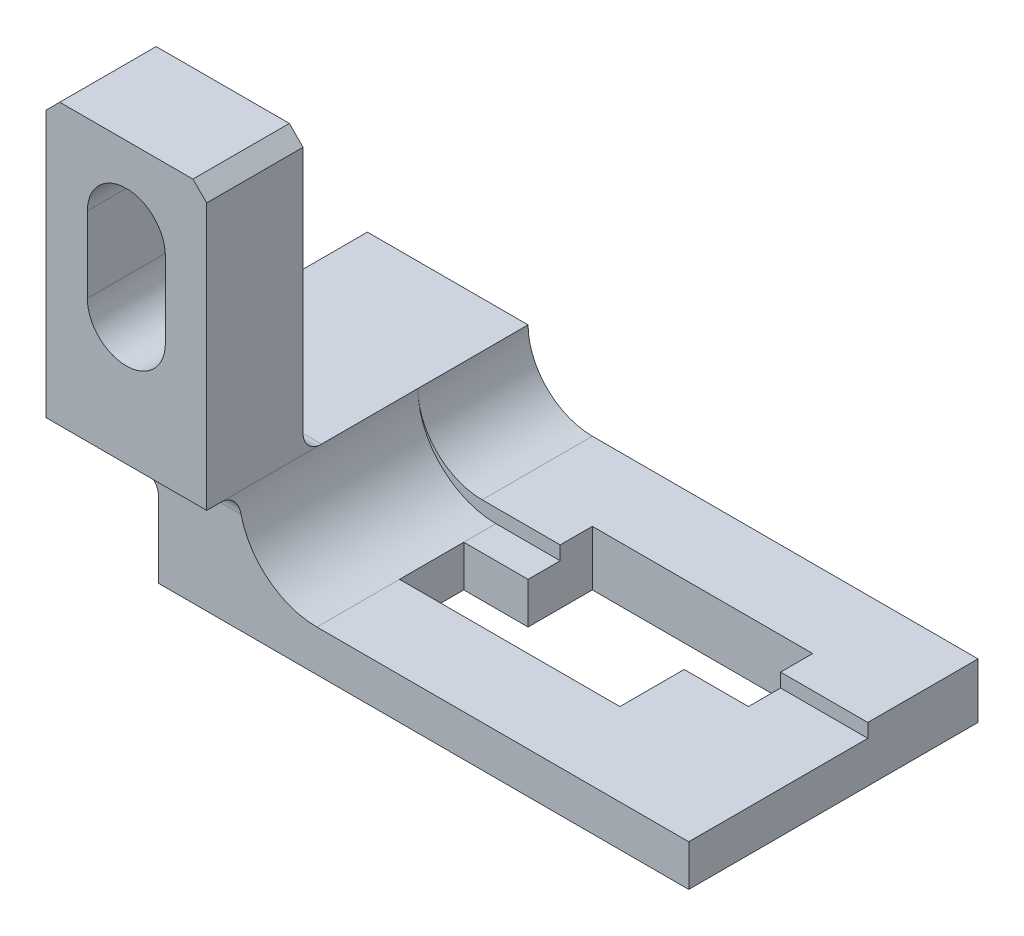
ISO-10303-21;
HEADER;
FILE_DESCRIPTION(('STEP AP214'),'2;1');
FILE_NAME('part.step','',(''),(''),'','','');
FILE_SCHEMA(('AUTOMOTIVE_DESIGN { 1 0 10303 214 1 1 1 1 }'));
ENDSEC;
DATA;
#1=APPLICATION_CONTEXT('core data for automotive mechanical design processes');
#2=APPLICATION_PROTOCOL_DEFINITION('international standard','automotive_design',2000,#1);
#3=PRODUCT_CONTEXT('',#1,'mechanical');
#4=PRODUCT('Part','Part','',(#3));
#5=PRODUCT_RELATED_PRODUCT_CATEGORY('part','',(#4));
#6=PRODUCT_DEFINITION_FORMATION('','',#4);
#7=PRODUCT_DEFINITION_CONTEXT('part definition',#1,'design');
#8=PRODUCT_DEFINITION('design','',#6,#7);
#9=PRODUCT_DEFINITION_SHAPE('','',#8);
#10=(LENGTH_UNIT() NAMED_UNIT(*) SI_UNIT(.MILLI.,.METRE.));
#11=(NAMED_UNIT(*) PLANE_ANGLE_UNIT() SI_UNIT($,.RADIAN.));
#12=(NAMED_UNIT(*) SI_UNIT($,.STERADIAN.) SOLID_ANGLE_UNIT());
#13=UNCERTAINTY_MEASURE_WITH_UNIT(LENGTH_MEASURE(1.E-05),#10,'distance_accuracy_value','');
#14=(GEOMETRIC_REPRESENTATION_CONTEXT(3) GLOBAL_UNCERTAINTY_ASSIGNED_CONTEXT((#13)) GLOBAL_UNIT_ASSIGNED_CONTEXT((#10,
#11,#12)) REPRESENTATION_CONTEXT('',''));
#15=CARTESIAN_POINT('',(0.,0.,0.));
#16=DIRECTION('',(0.,0.,1.));
#17=DIRECTION('',(1.,0.,0.));
#18=AXIS2_PLACEMENT_3D('',#15,#16,#17);
#19=CARTESIAN_POINT('',(0.,0.,31.5));
#20=DIRECTION('',(0.,-1.,0.));
#21=DIRECTION('',(0.,0.,-1.));
#22=AXIS2_PLACEMENT_3D('',#19,#20,#21);
#23=PLANE('',#22);
#24=DIRECTION('',(0.,0.,-1.));
#25=VECTOR('',#24,1.);
#26=CARTESIAN_POINT('',(0.,0.,31.5));
#27=LINE('',#26,#25);
#28=CARTESIAN_POINT('',(0.,0.,13.5));
#29=VERTEX_POINT('',#28);
#30=CARTESIAN_POINT('',(0.,0.,-31.5));
#31=VERTEX_POINT('',#30);
#32=EDGE_CURVE('E438',#29,#31,#27,.T.);
#33=ORIENTED_EDGE('',*,*,#32,.F.);
#34=DIRECTION('',(-1.,0.,0.));
#35=VECTOR('',#34,1.);
#36=CARTESIAN_POINT('',(0.,0.,13.5));
#37=LINE('',#36,#35);
#38=CARTESIAN_POINT('',(35.,0.,13.5));
#39=VERTEX_POINT('',#38);
#40=EDGE_CURVE('E507',#29,#39,#37,.F.);
#41=ORIENTED_EDGE('',*,*,#40,.T.);
#42=DIRECTION('',(0.,0.,-1.));
#43=VECTOR('',#42,1.);
#44=CARTESIAN_POINT('',(35.,0.,31.5));
#45=LINE('',#44,#43);
#46=CARTESIAN_POINT('',(35.,0.,-7.5));
#47=VERTEX_POINT('',#46);
#48=EDGE_CURVE('E467',#39,#47,#45,.T.);
#49=ORIENTED_EDGE('',*,*,#48,.T.);
#50=CARTESIAN_POINT('',(35.,0.,-31.5));
#51=VERTEX_POINT('',#50);
#52=EDGE_CURVE('E462',#47,#51,#45,.T.);
#53=ORIENTED_EDGE('',*,*,#52,.T.);
#54=DIRECTION('',(-1.,0.,0.));
#55=VECTOR('',#54,1.);
#56=CARTESIAN_POINT('',(0.,0.,-31.5));
#57=LINE('',#56,#55);
#58=EDGE_CURVE('E428',#51,#31,#57,.T.);
#59=ORIENTED_EDGE('',*,*,#58,.T.);
#60=EDGE_LOOP('',(#33,#41,#49,#53,#59));
#61=FACE_BOUND('',#60,.T.);
#62=ADVANCED_FACE('F41',(#61),#23,.F.);
#63=CARTESIAN_POINT('',(133.,-17.,-7.5));
#64=DIRECTION('',(0.,-1.,0.));
#65=DIRECTION('',(1.,0.,0.));
#66=AXIS2_PLACEMENT_3D('',#63,#64,#65);
#67=PLANE('',#66);
#68=DIRECTION('',(-1.,0.,0.));
#69=VECTOR('',#68,1.);
#70=CARTESIAN_POINT('',(52.,-17.,-0.49999999999999));
#71=LINE('',#70,#69);
#72=CARTESIAN_POINT('',(66.,-17.,-0.499999999999991));
#73=VERTEX_POINT('',#72);
#74=CARTESIAN_POINT('',(52.,-17.,-0.49999999999999));
#75=VERTEX_POINT('',#74);
#76=EDGE_CURVE('E340',#73,#75,#71,.T.);
#77=ORIENTED_EDGE('',*,*,#76,.F.);
#78=DIRECTION('',(0.,0.,1.));
#79=VECTOR('',#78,1.);
#80=CARTESIAN_POINT('',(66.,-17.,-0.499999999999991));
#81=LINE('',#80,#79);
#82=CARTESIAN_POINT('',(66.,-17.,-7.5));
#83=VERTEX_POINT('',#82);
#84=EDGE_CURVE('E339',#83,#73,#81,.T.);
#85=ORIENTED_EDGE('',*,*,#84,.F.);
#86=DIRECTION('',(1.,0.,0.));
#87=VECTOR('',#86,1.);
#88=CARTESIAN_POINT('',(133.,-17.,-7.5));
#89=LINE('',#88,#87);
#90=CARTESIAN_POINT('',(52.,-17.,-7.5));
#91=VERTEX_POINT('',#90);
#92=EDGE_CURVE('E414',#91,#83,#89,.T.);
#93=ORIENTED_EDGE('',*,*,#92,.F.);
#94=DIRECTION('',(0.,0.,1.));
#95=VECTOR('',#94,1.);
#96=CARTESIAN_POINT('',(52.,-17.,-7.5));
#97=LINE('',#96,#95);
#98=EDGE_CURVE('E425',#91,#75,#97,.T.);
#99=ORIENTED_EDGE('',*,*,#98,.T.);
#100=EDGE_LOOP('',(#77,#85,#93,#99));
#101=FACE_BOUND('',#100,.T.);
#102=ADVANCED_FACE('F586',(#101),#67,.F.);
#103=CARTESIAN_POINT('',(49.,0.,-7.5));
#104=DIRECTION('',(0.,0.,1.));
#105=DIRECTION('',(1.,0.,0.));
#106=AXIS2_PLACEMENT_3D('',#103,#104,#105);
#107=PLANE('',#106);
#108=DIRECTION('',(0.,1.,0.));
#109=VECTOR('',#108,1.);
#110=CARTESIAN_POINT('',(66.,-26.001,-7.5));
#111=LINE('',#110,#109);
#112=CARTESIAN_POINT('',(66.,-14.,-7.5));
#113=VERTEX_POINT('',#112);
#114=EDGE_CURVE('E330',#83,#113,#111,.T.);
#115=ORIENTED_EDGE('',*,*,#114,.T.);
#116=DIRECTION('',(-1.,0.,0.));
#117=VECTOR('',#116,1.);
#118=CARTESIAN_POINT('',(133.,-14.,-7.5));
#119=LINE('',#118,#117);
#120=CARTESIAN_POINT('',(49.,-14.,-7.5));
#121=VERTEX_POINT('',#120);
#122=EDGE_CURVE('E398',#113,#121,#119,.T.);
#123=ORIENTED_EDGE('',*,*,#122,.T.);
#124=CARTESIAN_POINT('',(49.,0.,-7.5));
#125=DIRECTION('',(0.,0.,-1.));
#126=DIRECTION('',(1.,0.,0.));
#127=AXIS2_PLACEMENT_3D('',#124,#125,#126);
#128=CIRCLE('',#127,14.);
#129=EDGE_CURVE('E403',#121,#47,#128,.T.);
#130=ORIENTED_EDGE('',*,*,#129,.T.);
#131=CARTESIAN_POINT('',(52.,0.,-7.5));
#132=DIRECTION('',(0.,0.,1.));
#133=DIRECTION('',(-1.,0.,0.));
#134=AXIS2_PLACEMENT_3D('',#131,#132,#133);
#135=CIRCLE('',#134,17.);
#136=EDGE_CURVE('E409',#47,#91,#135,.T.);
#137=ORIENTED_EDGE('',*,*,#136,.T.);
#138=ORIENTED_EDGE('',*,*,#92,.T.);
#139=EDGE_LOOP('',(#115,#123,#130,#137,#138));
#140=FACE_BOUND('',#139,.T.);
#141=ADVANCED_FACE('F591',(#140),#107,.T.);
#142=CARTESIAN_POINT('',(49.,-14.,31.5));
#143=DIRECTION('',(0.,-1.,0.));
#144=DIRECTION('',(1.,0.,0.));
#145=AXIS2_PLACEMENT_3D('',#142,#143,#144);
#146=PLANE('',#145);
#147=ORIENTED_EDGE('',*,*,#122,.F.);
#148=DIRECTION('',(0.,0.,1.));
#149=VECTOR('',#148,1.);
#150=CARTESIAN_POINT('',(66.,-14.,-0.499999999999991));
#151=LINE('',#150,#149);
#152=CARTESIAN_POINT('',(66.,-14.,-14.5));
#153=VERTEX_POINT('',#152);
#154=EDGE_CURVE('E366',#153,#113,#151,.T.);
#155=ORIENTED_EDGE('',*,*,#154,.F.);
#156=DIRECTION('',(-1.,0.,0.));
#157=VECTOR('',#156,1.);
#158=CARTESIAN_POINT('',(66.,-14.,-14.5));
#159=LINE('',#158,#157);
#160=CARTESIAN_POINT('',(114.,-14.,-14.5));
#161=VERTEX_POINT('',#160);
#162=EDGE_CURVE('E364',#161,#153,#159,.T.);
#163=ORIENTED_EDGE('',*,*,#162,.F.);
#164=DIRECTION('',(0.,0.,-1.));
#165=VECTOR('',#164,1.);
#166=CARTESIAN_POINT('',(114.,-14.,-14.5));
#167=LINE('',#166,#165);
#168=CARTESIAN_POINT('',(114.,-14.,-7.5));
#169=VERTEX_POINT('',#168);
#170=EDGE_CURVE('E362',#169,#161,#167,.T.);
#171=ORIENTED_EDGE('',*,*,#170,.F.);
#172=CARTESIAN_POINT('',(133.,-14.,-7.5));
#173=VERTEX_POINT('',#172);
#174=EDGE_CURVE('E405',#173,#169,#119,.T.);
#175=ORIENTED_EDGE('',*,*,#174,.F.);
#176=DIRECTION('',(0.,0.,-1.));
#177=VECTOR('',#176,1.);
#178=CARTESIAN_POINT('',(133.,-14.,31.5));
#179=LINE('',#178,#177);
#180=CARTESIAN_POINT('',(133.,-14.,-31.5));
#181=VERTEX_POINT('',#180);
#182=EDGE_CURVE('E470',#173,#181,#179,.T.);
#183=ORIENTED_EDGE('',*,*,#182,.T.);
#184=DIRECTION('',(-1.,0.,0.));
#185=VECTOR('',#184,1.);
#186=CARTESIAN_POINT('',(49.,-14.,-31.5));
#187=LINE('',#186,#185);
#188=CARTESIAN_POINT('',(49.,-14.,-31.5));
#189=VERTEX_POINT('',#188);
#190=EDGE_CURVE('E455',#181,#189,#187,.T.);
#191=ORIENTED_EDGE('',*,*,#190,.T.);
#192=DIRECTION('',(0.,0.,-1.));
#193=VECTOR('',#192,1.);
#194=CARTESIAN_POINT('',(49.,-14.,31.5));
#195=LINE('',#194,#193);
#196=EDGE_CURVE('E465',#121,#189,#195,.T.);
#197=ORIENTED_EDGE('',*,*,#196,.F.);
#198=EDGE_LOOP('',(#147,#155,#163,#171,#175,#183,#191,#197));
#199=FACE_BOUND('',#198,.T.);
#200=ADVANCED_FACE('F557',(#199),#146,.F.);
#201=CARTESIAN_POINT('',(49.,0.,31.5));
#202=DIRECTION('',(0.,0.,-1.));
#203=DIRECTION('',(-1.,0.,0.));
#204=AXIS2_PLACEMENT_3D('',#201,#202,#203);
#205=CYLINDRICAL_SURFACE('',#204,14.);
#206=ORIENTED_EDGE('',*,*,#129,.F.);
#207=ORIENTED_EDGE('',*,*,#196,.T.);
#208=CARTESIAN_POINT('',(49.,0.,-31.5));
#209=DIRECTION('',(0.,0.,-1.));
#210=DIRECTION('',(1.,0.,0.));
#211=AXIS2_PLACEMENT_3D('',#208,#209,#210);
#212=CIRCLE('',#211,14.);
#213=EDGE_CURVE('E457',#189,#51,#212,.T.);
#214=ORIENTED_EDGE('',*,*,#213,.T.);
#215=ORIENTED_EDGE('',*,*,#52,.F.);
#216=EDGE_LOOP('',(#206,#207,#214,#215));
#217=FACE_BOUND('',#216,.T.);
#218=ADVANCED_FACE('F648',(#217),#205,.F.);
#219=CARTESIAN_POINT('',(0.,0.,31.5));
#220=DIRECTION('',(1.,0.,0.));
#221=DIRECTION('',(0.,1.,0.));
#222=AXIS2_PLACEMENT_3D('',#219,#220,#221);
#223=PLANE('',#222);
#224=DIRECTION('',(0.,1.,0.));
#225=VECTOR('',#224,1.);
#226=CARTESIAN_POINT('',(0.,0.,38.5));
#227=LINE('',#226,#225);
#228=CARTESIAN_POINT('',(0.,0.,38.5));
#229=VERTEX_POINT('',#228);
#230=CARTESIAN_POINT('',(0.,58.,38.5));
#231=VERTEX_POINT('',#230);
#232=EDGE_CURVE('E301',#229,#231,#227,.T.);
#233=ORIENTED_EDGE('',*,*,#232,.T.);
#234=DIRECTION('',(0.,0.,-1.));
#235=VECTOR('',#234,1.);
#236=CARTESIAN_POINT('',(0.,58.,17.5));
#237=LINE('',#236,#235);
#238=CARTESIAN_POINT('',(0.,58.,17.5));
#239=VERTEX_POINT('',#238);
#240=EDGE_CURVE('E484',#231,#239,#237,.T.);
#241=ORIENTED_EDGE('',*,*,#240,.T.);
#242=DIRECTION('',(0.,-1.,0.));
#243=VECTOR('',#242,1.);
#244=CARTESIAN_POINT('',(0.,61.,17.5));
#245=LINE('',#244,#243);
#246=CARTESIAN_POINT('',(0.,4.,17.5));
#247=VERTEX_POINT('',#246);
#248=EDGE_CURVE('E298',#239,#247,#245,.T.);
#249=ORIENTED_EDGE('',*,*,#248,.T.);
#250=CARTESIAN_POINT('',(0.,4.,13.5));
#251=DIRECTION('',(1.,0.,0.));
#252=DIRECTION('',(0.,1.,0.));
#253=AXIS2_PLACEMENT_3D('',#250,#251,#252);
#254=CIRCLE('',#253,4.);
#255=EDGE_CURVE('E513',#247,#29,#254,.T.);
#256=ORIENTED_EDGE('',*,*,#255,.T.);
#257=ORIENTED_EDGE('',*,*,#32,.T.);
#258=DIRECTION('',(0.,-1.,0.));
#259=VECTOR('',#258,1.);
#260=CARTESIAN_POINT('',(0.,0.,-31.5));
#261=LINE('',#260,#259);
#262=CARTESIAN_POINT('',(0.,-6.,-31.5));
#263=VERTEX_POINT('',#262);
#264=EDGE_CURVE('E423',#31,#263,#261,.T.);
#265=ORIENTED_EDGE('',*,*,#264,.T.);
#266=DIRECTION('',(0.,0.,-1.));
#267=VECTOR('',#266,1.);
#268=CARTESIAN_POINT('',(0.,-6.,31.5));
#269=LINE('',#268,#267);
#270=CARTESIAN_POINT('',(0.,-6.,31.5));
#271=VERTEX_POINT('',#270);
#272=EDGE_CURVE('E485',#271,#263,#269,.T.);
#273=ORIENTED_EDGE('',*,*,#272,.F.);
#274=DIRECTION('',(0.,-1.,0.));
#275=VECTOR('',#274,1.);
#276=CARTESIAN_POINT('',(0.,0.,31.5));
#277=LINE('',#276,#275);
#278=CARTESIAN_POINT('',(0.,-4.,31.5));
#279=VERTEX_POINT('',#278);
#280=EDGE_CURVE('E422',#279,#271,#277,.T.);
#281=ORIENTED_EDGE('',*,*,#280,.F.);
#282=CARTESIAN_POINT('',(0.,-4.,35.5));
#283=DIRECTION('',(1.,0.,0.));
#284=DIRECTION('',(0.,1.,0.));
#285=AXIS2_PLACEMENT_3D('',#282,#283,#284);
#286=CIRCLE('',#285,4.);
#287=CARTESIAN_POINT('',(0.,0.,35.5));
#288=VERTEX_POINT('',#287);
#289=EDGE_CURVE('E54',#279,#288,#286,.T.);
#290=ORIENTED_EDGE('',*,*,#289,.T.);
#291=DIRECTION('',(0.,0.,1.));
#292=VECTOR('',#291,1.);
#293=CARTESIAN_POINT('',(0.,0.,17.5));
#294=LINE('',#293,#292);
#295=EDGE_CURVE('E315',#288,#229,#294,.T.);
#296=ORIENTED_EDGE('',*,*,#295,.T.);
#297=EDGE_LOOP('',(#233,#241,#249,#256,#257,#265,#273,#281,#290,#296));
#298=FACE_BOUND('',#297,.T.);
#299=ADVANCED_FACE('F522',(#298),#223,.F.);
#300=CARTESIAN_POINT('',(0.,-6.,31.5));
#301=DIRECTION('',(0.,1.,0.));
#302=DIRECTION('',(0.,0.,1.));
#303=AXIS2_PLACEMENT_3D('',#300,#301,#302);
#304=PLANE('',#303);
#305=DIRECTION('',(1.,0.,0.));
#306=VECTOR('',#305,1.);
#307=CARTESIAN_POINT('',(0.,-6.,-31.5));
#308=LINE('',#307,#306);
#309=CARTESIAN_POINT('',(14.,-6.,-31.5));
#310=VERTEX_POINT('',#309);
#311=EDGE_CURVE('E445',#263,#310,#308,.T.);
#312=ORIENTED_EDGE('',*,*,#311,.T.);
#313=DIRECTION('',(0.,0.,-1.));
#314=VECTOR('',#313,1.);
#315=CARTESIAN_POINT('',(14.,-6.,31.5));
#316=LINE('',#315,#314);
#317=CARTESIAN_POINT('',(14.,-6.,31.5));
#318=VERTEX_POINT('',#317);
#319=EDGE_CURVE('E479',#318,#310,#316,.T.);
#320=ORIENTED_EDGE('',*,*,#319,.F.);
#321=DIRECTION('',(1.,0.,0.));
#322=VECTOR('',#321,1.);
#323=CARTESIAN_POINT('',(0.,-6.,31.5));
#324=LINE('',#323,#322);
#325=EDGE_CURVE('E430',#271,#318,#324,.T.);
#326=ORIENTED_EDGE('',*,*,#325,.F.);
#327=ORIENTED_EDGE('',*,*,#272,.T.);
#328=EDGE_LOOP('',(#312,#320,#326,#327));
#329=FACE_BOUND('',#328,.T.);
#330=ADVANCED_FACE('F630',(#329),#304,.F.);
#331=CARTESIAN_POINT('',(14.,-9.5,31.5));
#332=DIRECTION('',(0.,0.,-1.));
#333=DIRECTION('',(-1.,0.,0.));
#334=AXIS2_PLACEMENT_3D('',#331,#332,#333);
#335=CYLINDRICAL_SURFACE('',#334,3.5);
#336=CARTESIAN_POINT('',(14.,-9.5,-31.5));
#337=DIRECTION('',(0.,0.,-1.));
#338=DIRECTION('',(-1.,0.,0.));
#339=AXIS2_PLACEMENT_3D('',#336,#337,#338);
#340=CIRCLE('',#339,3.5);
#341=CARTESIAN_POINT('',(17.5,-9.50000000000002,-31.5));
#342=VERTEX_POINT('',#341);
#343=EDGE_CURVE('E441',#310,#342,#340,.T.);
#344=ORIENTED_EDGE('',*,*,#343,.T.);
#345=DIRECTION('',(0.,0.,-1.));
#346=VECTOR('',#345,1.);
#347=CARTESIAN_POINT('',(17.5,-9.50000000000002,31.5));
#348=LINE('',#347,#346);
#349=CARTESIAN_POINT('',(17.5,-9.50000000000002,31.5));
#350=VERTEX_POINT('',#349);
#351=EDGE_CURVE('E478',#350,#342,#348,.T.);
#352=ORIENTED_EDGE('',*,*,#351,.F.);
#353=CARTESIAN_POINT('',(14.,-9.5,31.5));
#354=DIRECTION('',(0.,0.,-1.));
#355=DIRECTION('',(-1.,0.,0.));
#356=AXIS2_PLACEMENT_3D('',#353,#354,#355);
#357=CIRCLE('',#356,3.5);
#358=EDGE_CURVE('E429',#318,#350,#357,.T.);
#359=ORIENTED_EDGE('',*,*,#358,.F.);
#360=ORIENTED_EDGE('',*,*,#319,.T.);
#361=EDGE_LOOP('',(#344,#352,#359,#360));
#362=FACE_BOUND('',#361,.T.);
#363=ADVANCED_FACE('F637',(#362),#335,.F.);
#364=CARTESIAN_POINT('',(17.5,-9.50000000000002,31.5));
#365=DIRECTION('',(1.,0.,0.));
#366=DIRECTION('',(0.,1.,0.));
#367=AXIS2_PLACEMENT_3D('',#364,#365,#366);
#368=PLANE('',#367);
#369=DIRECTION('',(0.,-1.,0.));
#370=VECTOR('',#369,1.);
#371=CARTESIAN_POINT('',(17.5,-9.50000000000002,-31.5));
#372=LINE('',#371,#370);
#373=CARTESIAN_POINT('',(17.5,-26.,-31.5));
#374=VERTEX_POINT('',#373);
#375=EDGE_CURVE('E446',#342,#374,#372,.T.);
#376=ORIENTED_EDGE('',*,*,#375,.T.);
#377=DIRECTION('',(0.,0.,-1.));
#378=VECTOR('',#377,1.);
#379=CARTESIAN_POINT('',(17.5,-26.,31.5));
#380=LINE('',#379,#378);
#381=CARTESIAN_POINT('',(17.5,-26.,31.5));
#382=VERTEX_POINT('',#381);
#383=EDGE_CURVE('E471',#382,#374,#380,.T.);
#384=ORIENTED_EDGE('',*,*,#383,.F.);
#385=DIRECTION('',(0.,-1.,0.));
#386=VECTOR('',#385,1.);
#387=CARTESIAN_POINT('',(17.5,-9.50000000000002,31.5));
#388=LINE('',#387,#386);
#389=EDGE_CURVE('E435',#350,#382,#388,.T.);
#390=ORIENTED_EDGE('',*,*,#389,.F.);
#391=ORIENTED_EDGE('',*,*,#351,.T.);
#392=EDGE_LOOP('',(#376,#384,#390,#391));
#393=FACE_BOUND('',#392,.T.);
#394=ADVANCED_FACE('F639',(#393),#368,.F.);
#395=CARTESIAN_POINT('',(133.,-26.,31.5));
#396=DIRECTION('',(0.,1.,0.));
#397=DIRECTION('',(0.,0.,1.));
#398=AXIS2_PLACEMENT_3D('',#395,#396,#397);
#399=PLANE('',#398);
#400=DIRECTION('',(0.,0.,-1.));
#401=VECTOR('',#400,1.);
#402=CARTESIAN_POINT('',(66.,-26.,-0.499999999999991));
#403=LINE('',#402,#401);
#404=CARTESIAN_POINT('',(66.,-26.,-0.499999999999991));
#405=VERTEX_POINT('',#404);
#406=CARTESIAN_POINT('',(66.,-26.,-14.5));
#407=VERTEX_POINT('',#406);
#408=EDGE_CURVE('E357',#405,#407,#403,.T.);
#409=ORIENTED_EDGE('',*,*,#408,.F.);
#410=DIRECTION('',(1.,0.,0.));
#411=VECTOR('',#410,1.);
#412=CARTESIAN_POINT('',(52.,-26.,-0.49999999999999));
#413=LINE('',#412,#411);
#414=CARTESIAN_POINT('',(52.,-26.,-0.49999999999999));
#415=VERTEX_POINT('',#414);
#416=EDGE_CURVE('E356',#415,#405,#413,.T.);
#417=ORIENTED_EDGE('',*,*,#416,.F.);
#418=DIRECTION('',(0.,0.,-1.));
#419=VECTOR('',#418,1.);
#420=CARTESIAN_POINT('',(52.,-26.,13.5));
#421=LINE('',#420,#419);
#422=CARTESIAN_POINT('',(52.,-26.,13.5));
#423=VERTEX_POINT('',#422);
#424=EDGE_CURVE('E393',#423,#415,#421,.T.);
#425=ORIENTED_EDGE('',*,*,#424,.F.);
#426=DIRECTION('',(-1.,0.,0.));
#427=VECTOR('',#426,1.);
#428=CARTESIAN_POINT('',(100.,-26.,13.5));
#429=LINE('',#428,#427);
#430=CARTESIAN_POINT('',(100.,-26.,13.5));
#431=VERTEX_POINT('',#430);
#432=EDGE_CURVE('E344',#431,#423,#429,.T.);
#433=ORIENTED_EDGE('',*,*,#432,.F.);
#434=DIRECTION('',(0.,0.,1.));
#435=VECTOR('',#434,1.);
#436=CARTESIAN_POINT('',(100.,-26.,-0.499999999999997));
#437=LINE('',#436,#435);
#438=CARTESIAN_POINT('',(100.,-26.,-0.499999999999997));
#439=VERTEX_POINT('',#438);
#440=EDGE_CURVE('E343',#439,#431,#437,.T.);
#441=ORIENTED_EDGE('',*,*,#440,.F.);
#442=DIRECTION('',(-1.,0.,0.));
#443=VECTOR('',#442,1.);
#444=CARTESIAN_POINT('',(114.,-26.,-0.499999999999999));
#445=LINE('',#444,#443);
#446=CARTESIAN_POINT('',(114.,-26.,-0.499999999999999));
#447=VERTEX_POINT('',#446);
#448=EDGE_CURVE('E350',#447,#439,#445,.T.);
#449=ORIENTED_EDGE('',*,*,#448,.F.);
#450=DIRECTION('',(0.,0.,1.));
#451=VECTOR('',#450,1.);
#452=CARTESIAN_POINT('',(114.,-26.,-14.5));
#453=LINE('',#452,#451);
#454=CARTESIAN_POINT('',(114.,-26.,-14.5));
#455=VERTEX_POINT('',#454);
#456=EDGE_CURVE('E348',#455,#447,#453,.T.);
#457=ORIENTED_EDGE('',*,*,#456,.F.);
#458=DIRECTION('',(1.,0.,0.));
#459=VECTOR('',#458,1.);
#460=CARTESIAN_POINT('',(66.,-26.,-14.5));
#461=LINE('',#460,#459);
#462=EDGE_CURVE('E354',#407,#455,#461,.T.);
#463=ORIENTED_EDGE('',*,*,#462,.F.);
#464=EDGE_LOOP('',(#409,#417,#425,#433,#441,#449,#457,#463));
#465=FACE_BOUND('',#464,.T.);
#466=DIRECTION('',(1.,0.,0.));
#467=VECTOR('',#466,1.);
#468=CARTESIAN_POINT('',(133.,-26.,-31.5));
#469=LINE('',#468,#467);
#470=CARTESIAN_POINT('',(133.,-26.,-31.5));
#471=VERTEX_POINT('',#470);
#472=EDGE_CURVE('E449',#374,#471,#469,.T.);
#473=ORIENTED_EDGE('',*,*,#472,.T.);
#474=DIRECTION('',(0.,0.,-1.));
#475=VECTOR('',#474,1.);
#476=CARTESIAN_POINT('',(133.,-26.,31.5));
#477=LINE('',#476,#475);
#478=CARTESIAN_POINT('',(133.,-26.,31.5));
#479=VERTEX_POINT('',#478);
#480=EDGE_CURVE('E468',#479,#471,#477,.T.);
#481=ORIENTED_EDGE('',*,*,#480,.F.);
#482=DIRECTION('',(1.,0.,0.));
#483=VECTOR('',#482,1.);
#484=CARTESIAN_POINT('',(133.,-26.,31.5));
#485=LINE('',#484,#483);
#486=EDGE_CURVE('E432',#382,#479,#485,.T.);
#487=ORIENTED_EDGE('',*,*,#486,.F.);
#488=ORIENTED_EDGE('',*,*,#383,.T.);
#489=EDGE_LOOP('',(#473,#481,#487,#488));
#490=FACE_BOUND('',#489,.T.);
#491=ADVANCED_FACE('F574',(#465,#490),#399,.F.);
#492=CARTESIAN_POINT('',(133.,-14.,31.5));
#493=DIRECTION('',(-1.,0.,0.));
#494=DIRECTION('',(0.,0.,1.));
#495=AXIS2_PLACEMENT_3D('',#492,#493,#494);
#496=PLANE('',#495);
#497=DIRECTION('',(0.,1.,0.));
#498=VECTOR('',#497,1.);
#499=CARTESIAN_POINT('',(133.,-17.,-7.5));
#500=LINE('',#499,#498);
#501=CARTESIAN_POINT('',(133.,-17.,-7.5));
#502=VERTEX_POINT('',#501);
#503=EDGE_CURVE('E400',#502,#173,#500,.T.);
#504=ORIENTED_EDGE('',*,*,#503,.F.);
#505=DIRECTION('',(0.,0.,1.));
#506=VECTOR('',#505,1.);
#507=CARTESIAN_POINT('',(133.,-17.,-7.5));
#508=LINE('',#507,#506);
#509=CARTESIAN_POINT('',(133.,-17.,31.5));
#510=VERTEX_POINT('',#509);
#511=EDGE_CURVE('E416',#502,#510,#508,.T.);
#512=ORIENTED_EDGE('',*,*,#511,.T.);
#513=DIRECTION('',(0.,1.,0.));
#514=VECTOR('',#513,1.);
#515=CARTESIAN_POINT('',(133.,-14.,31.5));
#516=LINE('',#515,#514);
#517=EDGE_CURVE('E436',#479,#510,#516,.T.);
#518=ORIENTED_EDGE('',*,*,#517,.F.);
#519=ORIENTED_EDGE('',*,*,#480,.T.);
#520=DIRECTION('',(0.,1.,0.));
#521=VECTOR('',#520,1.);
#522=CARTESIAN_POINT('',(133.,-14.,-31.5));
#523=LINE('',#522,#521);
#524=EDGE_CURVE('E450',#471,#181,#523,.T.);
#525=ORIENTED_EDGE('',*,*,#524,.T.);
#526=ORIENTED_EDGE('',*,*,#182,.F.);
#527=EDGE_LOOP('',(#504,#512,#518,#519,#525,#526));
#528=FACE_BOUND('',#527,.T.);
#529=ADVANCED_FACE('F548',(#528),#496,.F.);
#530=CARTESIAN_POINT('',(14.,-9.5,31.5));
#531=DIRECTION('',(0.,0.,-1.));
#532=DIRECTION('',(-1.,0.,0.));
#533=AXIS2_PLACEMENT_3D('',#530,#531,#532);
#534=PLANE('',#533);
#535=CARTESIAN_POINT('',(52.,0.,31.5));
#536=DIRECTION('',(0.,0.,1.));
#537=DIRECTION('',(-1.,0.,0.));
#538=AXIS2_PLACEMENT_3D('',#535,#536,#537);
#539=CIRCLE('',#538,17.);
#540=CARTESIAN_POINT('',(35.4772883581417,-4.,31.5));
#541=VERTEX_POINT('',#540);
#542=CARTESIAN_POINT('',(52.,-17.,31.5));
#543=VERTEX_POINT('',#542);
#544=EDGE_CURVE('E399',#541,#543,#539,.T.);
#545=ORIENTED_EDGE('',*,*,#544,.F.);
#546=DIRECTION('',(-1.,0.,0.));
#547=VECTOR('',#546,1.);
#548=CARTESIAN_POINT('',(14.,-4.,31.5));
#549=LINE('',#548,#547);
#550=EDGE_CURVE('E506',#541,#279,#549,.T.);
#551=ORIENTED_EDGE('',*,*,#550,.T.);
#552=ORIENTED_EDGE('',*,*,#280,.T.);
#553=ORIENTED_EDGE('',*,*,#325,.T.);
#554=ORIENTED_EDGE('',*,*,#358,.T.);
#555=ORIENTED_EDGE('',*,*,#389,.T.);
#556=ORIENTED_EDGE('',*,*,#486,.T.);
#557=ORIENTED_EDGE('',*,*,#517,.T.);
#558=DIRECTION('',(1.,0.,0.));
#559=VECTOR('',#558,1.);
#560=CARTESIAN_POINT('',(133.,-17.,31.5));
#561=LINE('',#560,#559);
#562=EDGE_CURVE('E402',#543,#510,#561,.T.);
#563=ORIENTED_EDGE('',*,*,#562,.F.);
#564=EDGE_LOOP('',(#545,#551,#552,#553,#554,#555,#556,#557,#563));
#565=FACE_BOUND('',#564,.T.);
#566=ADVANCED_FACE('F539',(#565),#534,.F.);
#567=CARTESIAN_POINT('',(14.,-9.5,-31.5));
#568=DIRECTION('',(0.,0.,-1.));
#569=DIRECTION('',(-1.,0.,0.));
#570=AXIS2_PLACEMENT_3D('',#567,#568,#569);
#571=PLANE('',#570);
#572=ORIENTED_EDGE('',*,*,#264,.F.);
#573=ORIENTED_EDGE('',*,*,#58,.F.);
#574=ORIENTED_EDGE('',*,*,#213,.F.);
#575=ORIENTED_EDGE('',*,*,#190,.F.);
#576=ORIENTED_EDGE('',*,*,#524,.F.);
#577=ORIENTED_EDGE('',*,*,#472,.F.);
#578=ORIENTED_EDGE('',*,*,#375,.F.);
#579=ORIENTED_EDGE('',*,*,#343,.F.);
#580=ORIENTED_EDGE('',*,*,#311,.F.);
#581=EDGE_LOOP('',(#572,#573,#574,#575,#576,#577,#578,#579,#580));
#582=FACE_BOUND('',#581,.T.);
#583=ADVANCED_FACE('F626',(#582),#571,.T.);
#584=CARTESIAN_POINT('',(114.,-17.,-7.5));
#585=VERTEX_POINT('',#584);
#586=EDGE_CURVE('E412',#585,#502,#89,.T.);
#587=ORIENTED_EDGE('',*,*,#586,.F.);
#588=DIRECTION('',(0.,0.,-1.));
#589=VECTOR('',#588,1.);
#590=CARTESIAN_POINT('',(114.,-17.,-14.5));
#591=LINE('',#590,#589);
#592=CARTESIAN_POINT('',(114.,-17.,-0.499999999999999));
#593=VERTEX_POINT('',#592);
#594=EDGE_CURVE('E336',#593,#585,#591,.T.);
#595=ORIENTED_EDGE('',*,*,#594,.F.);
#596=DIRECTION('',(1.,0.,0.));
#597=VECTOR('',#596,1.);
#598=CARTESIAN_POINT('',(114.,-17.,-0.499999999999999));
#599=LINE('',#598,#597);
#600=CARTESIAN_POINT('',(100.,-17.,-0.499999999999997));
#601=VERTEX_POINT('',#600);
#602=EDGE_CURVE('E331',#601,#593,#599,.T.);
#603=ORIENTED_EDGE('',*,*,#602,.F.);
#604=DIRECTION('',(0.,0.,-1.));
#605=VECTOR('',#604,1.);
#606=CARTESIAN_POINT('',(100.,-17.,-0.499999999999997));
#607=LINE('',#606,#605);
#608=CARTESIAN_POINT('',(100.,-17.,13.5));
#609=VERTEX_POINT('',#608);
#610=EDGE_CURVE('E335',#609,#601,#607,.T.);
#611=ORIENTED_EDGE('',*,*,#610,.F.);
#612=DIRECTION('',(1.,0.,0.));
#613=VECTOR('',#612,1.);
#614=CARTESIAN_POINT('',(100.,-17.,13.5));
#615=LINE('',#614,#613);
#616=CARTESIAN_POINT('',(52.,-17.,13.5));
#617=VERTEX_POINT('',#616);
#618=EDGE_CURVE('E329',#617,#609,#615,.T.);
#619=ORIENTED_EDGE('',*,*,#618,.F.);
#620=EDGE_CURVE('E413',#617,#543,#97,.T.);
#621=ORIENTED_EDGE('',*,*,#620,.T.);
#622=ORIENTED_EDGE('',*,*,#562,.T.);
#623=ORIENTED_EDGE('',*,*,#511,.F.);
#624=EDGE_LOOP('',(#587,#595,#603,#611,#619,#621,#622,#623));
#625=FACE_BOUND('',#624,.T.);
#626=ADVANCED_FACE('F544',(#625),#67,.F.);
#627=CARTESIAN_POINT('',(52.,0.,-7.5));
#628=DIRECTION('',(0.,0.,1.));
#629=DIRECTION('',(1.,0.,0.));
#630=AXIS2_PLACEMENT_3D('',#627,#628,#629);
#631=CYLINDRICAL_SURFACE('',#630,17.);
#632=CARTESIAN_POINT('',(35.,0.,35.5));
#633=VERTEX_POINT('',#632);
#634=EDGE_CURVE('E464',#633,#39,#45,.T.);
#635=ORIENTED_EDGE('',*,*,#634,.F.);
#636=CARTESIAN_POINT('',(35.,0.,35.5));
#637=CARTESIAN_POINT('',(35.0000083013039,1.07492089478438E-05,35.3875551600864));
#638=CARTESIAN_POINT('',(35.0000002164993,-0.00474140518274543,35.2751154336279));
#639=CARTESIAN_POINT('',(35.0000116692192,-0.0236883223681302,35.0510393368197));
#640=CARTESIAN_POINT('',(35.0000312054831,-0.0378826542354126,34.9394029300426));
#641=CARTESIAN_POINT('',(35.0001582427405,-0.0756183018738792,34.717789251689));
#642=CARTESIAN_POINT('',(35.0002656857482,-0.0991534509001617,34.6078109350756));
#643=CARTESIAN_POINT('',(35.0006870800331,-0.155379787783206,34.3902538389751));
#644=CARTESIAN_POINT('',(35.0010010287807,-0.188070863480572,34.2826750301115));
#645=CARTESIAN_POINT('',(35.002475089407,-0.299616249295769,33.9645689947982));
#646=CARTESIAN_POINT('',(35.0041672532816,-0.391956983501848,33.7585888256198));
#647=CARTESIAN_POINT('',(35.0105940252902,-0.609815982718297,33.3652251157232));
#648=CARTESIAN_POINT('',(35.0153281210827,-0.73532865860424,33.1778384495034));
#649=CARTESIAN_POINT('',(35.0297860201258,-1.01559300260569,32.8272621179482));
#650=CARTESIAN_POINT('',(35.039498240105,-1.17027626977358,32.6640174094866));
#651=CARTESIAN_POINT('',(35.0658728098731,-1.50444396712971,32.3659410961021));
#652=CARTESIAN_POINT('',(35.0825349222226,-1.68392754988818,32.2311085207306));
#653=CARTESIAN_POINT('',(35.1242644518129,-2.06034746483842,31.9947635630701));
#654=CARTESIAN_POINT('',(35.1492509862175,-2.25710292450681,31.8929484702819));
#655=CARTESIAN_POINT('',(35.2086941877631,-2.66348109747532,31.7234753466681));
#656=CARTESIAN_POINT('',(35.2431488829303,-2.87310112436463,31.6558102116013));
#657=CARTESIAN_POINT('',(35.310239320715,-3.23657295611819,31.5704717798367));
#658=CARTESIAN_POINT('',(35.3404773885729,-3.38886856149081,31.5439754018867));
#659=CARTESIAN_POINT('',(35.405514535937,-3.69427664557593,31.5087371885203));
#660=CARTESIAN_POINT('',(35.4403060702223,-3.84738737956684,31.4999663682107));
#661=CARTESIAN_POINT('',(35.4772883581417,-4.,31.5));
#662=B_SPLINE_CURVE_WITH_KNOTS('',3,(#636,#637,#638,#639,#640,#641,#642,#643,#644,#645,#646,
#647,#648,#649,#650,#651,#652,#653,#654,#655,#656,#657,#658,#659,#660,#661),.UNSPECIFIED.,.F.,
.F.,(4,2,2,2,2,2,2,2,2,2,2,2,4),(0.,0.337224909482972,0.674434429597278,1.01142169557896,
1.34840483367311,2.02212066534948,2.69572305525769,3.36776515140771,4.0397842894742,
4.70545556424118,5.37098830177873,5.8425107249983,6.31326148722317),.UNSPECIFIED.);
#663=EDGE_CURVE('E11',#633,#541,#662,.T.);
#664=ORIENTED_EDGE('',*,*,#663,.T.);
#665=ORIENTED_EDGE('',*,*,#544,.T.);
#666=ORIENTED_EDGE('',*,*,#620,.F.);
#667=DIRECTION('',(0.,0.,1.));
#668=VECTOR('',#667,1.);
#669=CARTESIAN_POINT('',(52.,-17.,-7.5));
#670=LINE('',#669,#668);
#671=EDGE_CURVE('E372',#75,#617,#670,.T.);
#672=ORIENTED_EDGE('',*,*,#671,.F.);
#673=ORIENTED_EDGE('',*,*,#98,.F.);
#674=ORIENTED_EDGE('',*,*,#136,.F.);
#675=ORIENTED_EDGE('',*,*,#48,.F.);
#676=EDGE_LOOP('',(#635,#664,#665,#666,#672,#673,#674,#675));
#677=FACE_BOUND('',#676,.T.);
#678=ADVANCED_FACE('F534',(#677),#631,.F.);
#679=DIRECTION('',(0.,-1.,0.));
#680=VECTOR('',#679,1.);
#681=CARTESIAN_POINT('',(114.,-26.001,-7.5));
#682=LINE('',#681,#680);
#683=EDGE_CURVE('E317',#169,#585,#682,.T.);
#684=ORIENTED_EDGE('',*,*,#683,.T.);
#685=ORIENTED_EDGE('',*,*,#586,.T.);
#686=ORIENTED_EDGE('',*,*,#503,.T.);
#687=ORIENTED_EDGE('',*,*,#174,.T.);
#688=EDGE_LOOP('',(#684,#685,#686,#687));
#689=FACE_BOUND('',#688,.T.);
#690=ADVANCED_FACE('F554',(#689),#107,.T.);
#691=CARTESIAN_POINT('',(66.,-26.001,-0.499999999999991));
#692=DIRECTION('',(-1.,0.,0.));
#693=DIRECTION('',(0.,-1.,0.));
#694=AXIS2_PLACEMENT_3D('',#691,#692,#693);
#695=PLANE('',#694);
#696=ORIENTED_EDGE('',*,*,#408,.T.);
#697=DIRECTION('',(0.,1.,0.));
#698=VECTOR('',#697,1.);
#699=CARTESIAN_POINT('',(66.,-26.001,-14.5));
#700=LINE('',#699,#698);
#701=EDGE_CURVE('E374',#407,#153,#700,.T.);
#702=ORIENTED_EDGE('',*,*,#701,.T.);
#703=ORIENTED_EDGE('',*,*,#154,.T.);
#704=ORIENTED_EDGE('',*,*,#114,.F.);
#705=ORIENTED_EDGE('',*,*,#84,.T.);
#706=DIRECTION('',(0.,1.,0.));
#707=VECTOR('',#706,1.);
#708=CARTESIAN_POINT('',(66.,-26.001,-0.499999999999991));
#709=LINE('',#708,#707);
#710=EDGE_CURVE('E371',#405,#73,#709,.T.);
#711=ORIENTED_EDGE('',*,*,#710,.F.);
#712=EDGE_LOOP('',(#696,#702,#703,#704,#705,#711));
#713=FACE_BOUND('',#712,.T.);
#714=ADVANCED_FACE('F673',(#713),#695,.F.);
#715=CARTESIAN_POINT('',(66.,-26.001,-14.5));
#716=DIRECTION('',(0.,0.,-1.));
#717=DIRECTION('',(-1.,0.,0.));
#718=AXIS2_PLACEMENT_3D('',#715,#716,#717);
#719=PLANE('',#718);
#720=ORIENTED_EDGE('',*,*,#462,.T.);
#721=DIRECTION('',(0.,1.,0.));
#722=VECTOR('',#721,1.);
#723=CARTESIAN_POINT('',(114.,-26.001,-14.5));
#724=LINE('',#723,#722);
#725=EDGE_CURVE('E380',#455,#161,#724,.T.);
#726=ORIENTED_EDGE('',*,*,#725,.T.);
#727=ORIENTED_EDGE('',*,*,#162,.T.);
#728=ORIENTED_EDGE('',*,*,#701,.F.);
#729=EDGE_LOOP('',(#720,#726,#727,#728));
#730=FACE_BOUND('',#729,.T.);
#731=ADVANCED_FACE('F693',(#730),#719,.F.);
#732=CARTESIAN_POINT('',(114.,-26.001,-14.5));
#733=DIRECTION('',(1.,0.,0.));
#734=DIRECTION('',(0.,1.,0.));
#735=AXIS2_PLACEMENT_3D('',#732,#733,#734);
#736=PLANE('',#735);
#737=ORIENTED_EDGE('',*,*,#456,.T.);
#738=DIRECTION('',(0.,1.,0.));
#739=VECTOR('',#738,1.);
#740=CARTESIAN_POINT('',(114.,-26.001,-0.499999999999999));
#741=LINE('',#740,#739);
#742=EDGE_CURVE('E377',#447,#593,#741,.T.);
#743=ORIENTED_EDGE('',*,*,#742,.T.);
#744=ORIENTED_EDGE('',*,*,#594,.T.);
#745=ORIENTED_EDGE('',*,*,#683,.F.);
#746=ORIENTED_EDGE('',*,*,#170,.T.);
#747=ORIENTED_EDGE('',*,*,#725,.F.);
#748=EDGE_LOOP('',(#737,#743,#744,#745,#746,#747));
#749=FACE_BOUND('',#748,.T.);
#750=ADVANCED_FACE('F562',(#749),#736,.F.);
#751=CARTESIAN_POINT('',(114.,-26.001,-0.499999999999999));
#752=DIRECTION('',(0.,0.,1.));
#753=DIRECTION('',(1.,0.,0.));
#754=AXIS2_PLACEMENT_3D('',#751,#752,#753);
#755=PLANE('',#754);
#756=ORIENTED_EDGE('',*,*,#448,.T.);
#757=DIRECTION('',(0.,1.,0.));
#758=VECTOR('',#757,1.);
#759=CARTESIAN_POINT('',(100.,-26.001,-0.499999999999997));
#760=LINE('',#759,#758);
#761=EDGE_CURVE('E385',#439,#601,#760,.T.);
#762=ORIENTED_EDGE('',*,*,#761,.T.);
#763=ORIENTED_EDGE('',*,*,#602,.T.);
#764=ORIENTED_EDGE('',*,*,#742,.F.);
#765=EDGE_LOOP('',(#756,#762,#763,#764));
#766=FACE_BOUND('',#765,.T.);
#767=ADVANCED_FACE('F567',(#766),#755,.F.);
#768=CARTESIAN_POINT('',(100.,-26.001,-0.499999999999997));
#769=DIRECTION('',(1.,0.,0.));
#770=DIRECTION('',(0.,1.,0.));
#771=AXIS2_PLACEMENT_3D('',#768,#769,#770);
#772=PLANE('',#771);
#773=ORIENTED_EDGE('',*,*,#440,.T.);
#774=DIRECTION('',(0.,1.,0.));
#775=VECTOR('',#774,1.);
#776=CARTESIAN_POINT('',(100.,-26.001,13.5));
#777=LINE('',#776,#775);
#778=EDGE_CURVE('E384',#431,#609,#777,.T.);
#779=ORIENTED_EDGE('',*,*,#778,.T.);
#780=ORIENTED_EDGE('',*,*,#610,.T.);
#781=ORIENTED_EDGE('',*,*,#761,.F.);
#782=EDGE_LOOP('',(#773,#779,#780,#781));
#783=FACE_BOUND('',#782,.T.);
#784=ADVANCED_FACE('F576',(#783),#772,.F.);
#785=CARTESIAN_POINT('',(52.,-26.001,13.5));
#786=DIRECTION('',(-1.,0.,0.));
#787=DIRECTION('',(0.,-1.,0.));
#788=AXIS2_PLACEMENT_3D('',#785,#786,#787);
#789=PLANE('',#788);
#790=ORIENTED_EDGE('',*,*,#424,.T.);
#791=DIRECTION('',(0.,1.,0.));
#792=VECTOR('',#791,1.);
#793=CARTESIAN_POINT('',(52.,-26.001,-0.49999999999999));
#794=LINE('',#793,#792);
#795=EDGE_CURVE('E367',#415,#75,#794,.T.);
#796=ORIENTED_EDGE('',*,*,#795,.T.);
#797=ORIENTED_EDGE('',*,*,#671,.T.);
#798=DIRECTION('',(0.,1.,0.));
#799=VECTOR('',#798,1.);
#800=CARTESIAN_POINT('',(52.,-26.001,13.5));
#801=LINE('',#800,#799);
#802=EDGE_CURVE('E389',#423,#617,#801,.T.);
#803=ORIENTED_EDGE('',*,*,#802,.F.);
#804=EDGE_LOOP('',(#790,#796,#797,#803));
#805=FACE_BOUND('',#804,.T.);
#806=ADVANCED_FACE('F679',(#805),#789,.F.);
#807=CARTESIAN_POINT('',(52.,-26.001,-0.49999999999999));
#808=DIRECTION('',(0.,0.,-1.));
#809=DIRECTION('',(-1.,0.,0.));
#810=AXIS2_PLACEMENT_3D('',#807,#808,#809);
#811=PLANE('',#810);
#812=ORIENTED_EDGE('',*,*,#416,.T.);
#813=ORIENTED_EDGE('',*,*,#710,.T.);
#814=ORIENTED_EDGE('',*,*,#76,.T.);
#815=ORIENTED_EDGE('',*,*,#795,.F.);
#816=EDGE_LOOP('',(#812,#813,#814,#815));
#817=FACE_BOUND('',#816,.T.);
#818=ADVANCED_FACE('F677',(#817),#811,.F.);
#819=CARTESIAN_POINT('',(100.,-26.001,13.5));
#820=DIRECTION('',(0.,0.,1.));
#821=DIRECTION('',(1.,0.,0.));
#822=AXIS2_PLACEMENT_3D('',#819,#820,#821);
#823=PLANE('',#822);
#824=ORIENTED_EDGE('',*,*,#432,.T.);
#825=ORIENTED_EDGE('',*,*,#802,.T.);
#826=ORIENTED_EDGE('',*,*,#618,.T.);
#827=ORIENTED_EDGE('',*,*,#778,.F.);
#828=EDGE_LOOP('',(#824,#825,#826,#827));
#829=FACE_BOUND('',#828,.T.);
#830=ADVANCED_FACE('F583',(#829),#823,.F.);
#831=CARTESIAN_POINT('',(35.,0.,17.5));
#832=DIRECTION('',(0.,-1.,0.));
#833=DIRECTION('',(1.,0.,0.));
#834=AXIS2_PLACEMENT_3D('',#831,#832,#833);
#835=PLANE('',#834);
#836=ORIENTED_EDGE('',*,*,#295,.F.);
#837=DIRECTION('',(-1.,0.,0.));
#838=VECTOR('',#837,1.);
#839=CARTESIAN_POINT('',(35.,0.,35.5));
#840=LINE('',#839,#838);
#841=EDGE_CURVE('E515',#288,#633,#840,.F.);
#842=ORIENTED_EDGE('',*,*,#841,.T.);
#843=DIRECTION('',(0.,0.,1.));
#844=VECTOR('',#843,1.);
#845=CARTESIAN_POINT('',(35.,0.,17.5));
#846=LINE('',#845,#844);
#847=CARTESIAN_POINT('',(35.,0.,38.5));
#848=VERTEX_POINT('',#847);
#849=EDGE_CURVE('E305',#633,#848,#846,.T.);
#850=ORIENTED_EDGE('',*,*,#849,.T.);
#851=DIRECTION('',(-1.,0.,0.));
#852=VECTOR('',#851,1.);
#853=CARTESIAN_POINT('',(35.,0.,38.5));
#854=LINE('',#853,#852);
#855=EDGE_CURVE('E310',#848,#229,#854,.T.);
#856=ORIENTED_EDGE('',*,*,#855,.T.);
#857=EDGE_LOOP('',(#836,#842,#850,#856));
#858=FACE_BOUND('',#857,.T.);
#859=ADVANCED_FACE('F527',(#858),#835,.T.);
#860=CARTESIAN_POINT('',(35.,61.,17.5));
#861=DIRECTION('',(0.,0.,-1.));
#862=DIRECTION('',(-1.,0.,0.));
#863=AXIS2_PLACEMENT_3D('',#860,#861,#862);
#864=PLANE('',#863);
#865=CARTESIAN_POINT('',(17.5,43.5,17.5));
#866=DIRECTION('',(0.,0.,-1.));
#867=DIRECTION('',(-1.,0.,0.));
#868=AXIS2_PLACEMENT_3D('',#865,#866,#867);
#869=CIRCLE('',#868,8.5);
#870=CARTESIAN_POINT('',(9.00000000000001,43.5,17.5));
#871=VERTEX_POINT('',#870);
#872=CARTESIAN_POINT('',(26.,43.5,17.5));
#873=VERTEX_POINT('',#872);
#874=EDGE_CURVE('E297',#871,#873,#869,.T.);
#875=ORIENTED_EDGE('',*,*,#874,.F.);
#876=DIRECTION('',(0.,1.,0.));
#877=VECTOR('',#876,1.);
#878=CARTESIAN_POINT('',(9.00000000000001,61.,17.5));
#879=LINE('',#878,#877);
#880=CARTESIAN_POINT('',(9.00000000000001,27.,17.5));
#881=VERTEX_POINT('',#880);
#882=EDGE_CURVE('E288',#881,#871,#879,.T.);
#883=ORIENTED_EDGE('',*,*,#882,.F.);
#884=CARTESIAN_POINT('',(17.5,27.,17.5));
#885=DIRECTION('',(0.,0.,-1.));
#886=DIRECTION('',(-1.,0.,0.));
#887=AXIS2_PLACEMENT_3D('',#884,#885,#886);
#888=CIRCLE('',#887,8.5);
#889=CARTESIAN_POINT('',(26.,27.,17.5));
#890=VERTEX_POINT('',#889);
#891=EDGE_CURVE('E269',#890,#881,#888,.T.);
#892=ORIENTED_EDGE('',*,*,#891,.F.);
#893=DIRECTION('',(0.,-1.,0.));
#894=VECTOR('',#893,1.);
#895=CARTESIAN_POINT('',(26.,61.,17.5));
#896=LINE('',#895,#894);
#897=EDGE_CURVE('E293',#873,#890,#896,.T.);
#898=ORIENTED_EDGE('',*,*,#897,.F.);
#899=EDGE_LOOP('',(#875,#883,#892,#898));
#900=FACE_BOUND('',#899,.T.);
#901=DIRECTION('',(0.,-1.,0.));
#902=VECTOR('',#901,1.);
#903=CARTESIAN_POINT('',(35.,61.,17.5));
#904=LINE('',#903,#902);
#905=CARTESIAN_POINT('',(35.,58.,17.5));
#906=VERTEX_POINT('',#905);
#907=CARTESIAN_POINT('',(35.,4.,17.5));
#908=VERTEX_POINT('',#907);
#909=EDGE_CURVE('E300',#906,#908,#904,.T.);
#910=ORIENTED_EDGE('',*,*,#909,.T.);
#911=DIRECTION('',(-1.,0.,0.));
#912=VECTOR('',#911,1.);
#913=CARTESIAN_POINT('',(35.,4.,17.5));
#914=LINE('',#913,#912);
#915=EDGE_CURVE('E504',#908,#247,#914,.T.);
#916=ORIENTED_EDGE('',*,*,#915,.T.);
#917=ORIENTED_EDGE('',*,*,#248,.F.);
#918=DIRECTION('',(0.707106781186549,0.707106781186546,0.));
#919=VECTOR('',#918,1.);
#920=CARTESIAN_POINT('',(19.0000000000001,77.,17.5));
#921=LINE('',#920,#919);
#922=CARTESIAN_POINT('',(2.99999999999998,61.,17.5));
#923=VERTEX_POINT('',#922);
#924=EDGE_CURVE('E489',#239,#923,#921,.T.);
#925=ORIENTED_EDGE('',*,*,#924,.T.);
#926=DIRECTION('',(-1.,0.,0.));
#927=VECTOR('',#926,1.);
#928=CARTESIAN_POINT('',(35.,61.,17.5));
#929=LINE('',#928,#927);
#930=CARTESIAN_POINT('',(32.,61.,17.5));
#931=VERTEX_POINT('',#930);
#932=EDGE_CURVE('E316',#931,#923,#929,.T.);
#933=ORIENTED_EDGE('',*,*,#932,.F.);
#934=DIRECTION('',(0.707106781186546,-0.707106781186549,0.));
#935=VECTOR('',#934,1.);
#936=CARTESIAN_POINT('',(33.5,59.5,17.5));
#937=LINE('',#936,#935);
#938=EDGE_CURVE('E488',#931,#906,#937,.T.);
#939=ORIENTED_EDGE('',*,*,#938,.T.);
#940=EDGE_LOOP('',(#910,#916,#917,#925,#933,#939));
#941=FACE_BOUND('',#940,.T.);
#942=ADVANCED_FACE('F604',(#900,#941),#864,.T.);
#943=CARTESIAN_POINT('',(35.,61.,17.5));
#944=DIRECTION('',(0.,1.,0.));
#945=DIRECTION('',(0.,0.,1.));
#946=AXIS2_PLACEMENT_3D('',#943,#944,#945);
#947=PLANE('',#946);
#948=ORIENTED_EDGE('',*,*,#932,.T.);
#949=DIRECTION('',(0.,0.,1.));
#950=VECTOR('',#949,1.);
#951=CARTESIAN_POINT('',(2.99999999999998,61.,38.5));
#952=LINE('',#951,#950);
#953=CARTESIAN_POINT('',(2.99999999999998,61.,38.5));
#954=VERTEX_POINT('',#953);
#955=EDGE_CURVE('E494',#923,#954,#952,.T.);
#956=ORIENTED_EDGE('',*,*,#955,.T.);
#957=DIRECTION('',(-1.,0.,0.));
#958=VECTOR('',#957,1.);
#959=CARTESIAN_POINT('',(35.,61.,38.5));
#960=LINE('',#959,#958);
#961=CARTESIAN_POINT('',(32.,61.,38.5));
#962=VERTEX_POINT('',#961);
#963=EDGE_CURVE('E319',#962,#954,#960,.T.);
#964=ORIENTED_EDGE('',*,*,#963,.F.);
#965=DIRECTION('',(0.,0.,-1.));
#966=VECTOR('',#965,1.);
#967=CARTESIAN_POINT('',(32.,61.,17.5));
#968=LINE('',#967,#966);
#969=EDGE_CURVE('E495',#962,#931,#968,.T.);
#970=ORIENTED_EDGE('',*,*,#969,.T.);
#971=EDGE_LOOP('',(#948,#956,#964,#970));
#972=FACE_BOUND('',#971,.T.);
#973=ADVANCED_FACE('F613',(#972),#947,.T.);
#974=CARTESIAN_POINT('',(35.,0.,38.5));
#975=DIRECTION('',(0.,0.,1.));
#976=DIRECTION('',(1.,0.,0.));
#977=AXIS2_PLACEMENT_3D('',#974,#975,#976);
#978=PLANE('',#977);
#979=CARTESIAN_POINT('',(17.5,43.5,38.5));
#980=DIRECTION('',(0.,0.,1.));
#981=DIRECTION('',(1.,0.,0.));
#982=AXIS2_PLACEMENT_3D('',#979,#980,#981);
#983=CIRCLE('',#982,8.5);
#984=CARTESIAN_POINT('',(26.,43.5,38.5));
#985=VERTEX_POINT('',#984);
#986=CARTESIAN_POINT('',(9.00000000000001,43.5,38.5));
#987=VERTEX_POINT('',#986);
#988=EDGE_CURVE('E68',#985,#987,#983,.T.);
#989=ORIENTED_EDGE('',*,*,#988,.F.);
#990=DIRECTION('',(0.,1.,0.));
#991=VECTOR('',#990,1.);
#992=CARTESIAN_POINT('',(26.,43.5,38.5));
#993=LINE('',#992,#991);
#994=CARTESIAN_POINT('',(26.,27.,38.5));
#995=VERTEX_POINT('',#994);
#996=EDGE_CURVE('E284',#995,#985,#993,.T.);
#997=ORIENTED_EDGE('',*,*,#996,.F.);
#998=CARTESIAN_POINT('',(17.5,27.,38.5));
#999=DIRECTION('',(0.,0.,1.));
#1000=DIRECTION('',(1.,0.,0.));
#1001=AXIS2_PLACEMENT_3D('',#998,#999,#1000);
#1002=CIRCLE('',#1001,8.5);
#1003=CARTESIAN_POINT('',(9.,27.,38.5));
#1004=VERTEX_POINT('',#1003);
#1005=EDGE_CURVE('E270',#1004,#995,#1002,.T.);
#1006=ORIENTED_EDGE('',*,*,#1005,.F.);
#1007=DIRECTION('',(0.,-1.,0.));
#1008=VECTOR('',#1007,1.);
#1009=CARTESIAN_POINT('',(9.00000000000001,43.5,38.5));
#1010=LINE('',#1009,#1008);
#1011=EDGE_CURVE('E277',#987,#1004,#1010,.T.);
#1012=ORIENTED_EDGE('',*,*,#1011,.F.);
#1013=EDGE_LOOP('',(#989,#997,#1006,#1012));
#1014=FACE_BOUND('',#1013,.T.);
#1015=ORIENTED_EDGE('',*,*,#963,.T.);
#1016=DIRECTION('',(-0.707106781186549,-0.707106781186546,0.));
#1017=VECTOR('',#1016,1.);
#1018=CARTESIAN_POINT('',(-11.4999999999999,46.5000000000001,38.5));
#1019=LINE('',#1018,#1017);
#1020=EDGE_CURVE('E496',#954,#231,#1019,.T.);
#1021=ORIENTED_EDGE('',*,*,#1020,.T.);
#1022=ORIENTED_EDGE('',*,*,#232,.F.);
#1023=ORIENTED_EDGE('',*,*,#855,.F.);
#1024=DIRECTION('',(0.,1.,0.));
#1025=VECTOR('',#1024,1.);
#1026=CARTESIAN_POINT('',(35.,0.,38.5));
#1027=LINE('',#1026,#1025);
#1028=CARTESIAN_POINT('',(35.,57.9999999999999,38.5));
#1029=VERTEX_POINT('',#1028);
#1030=EDGE_CURVE('E308',#848,#1029,#1027,.T.);
#1031=ORIENTED_EDGE('',*,*,#1030,.T.);
#1032=DIRECTION('',(-0.707106781186546,0.707106781186549,0.));
#1033=VECTOR('',#1032,1.);
#1034=CARTESIAN_POINT('',(64.,28.9999999999998,38.5));
#1035=LINE('',#1034,#1033);
#1036=EDGE_CURVE('E500',#1029,#962,#1035,.T.);
#1037=ORIENTED_EDGE('',*,*,#1036,.T.);
#1038=EDGE_LOOP('',(#1015,#1021,#1022,#1023,#1031,#1037));
#1039=FACE_BOUND('',#1038,.T.);
#1040=ADVANCED_FACE('F278',(#1014,#1039),#978,.T.);
#1041=CARTESIAN_POINT('',(35.,0.,0.));
#1042=DIRECTION('',(-1.,0.,0.));
#1043=DIRECTION('',(0.,-1.,0.));
#1044=AXIS2_PLACEMENT_3D('',#1041,#1042,#1043);
#1045=PLANE('',#1044);
#1046=ORIENTED_EDGE('',*,*,#909,.F.);
#1047=DIRECTION('',(0.,0.,1.));
#1048=VECTOR('',#1047,1.);
#1049=CARTESIAN_POINT('',(35.,58.,38.5));
#1050=LINE('',#1049,#1048);
#1051=EDGE_CURVE('E501',#906,#1029,#1050,.T.);
#1052=ORIENTED_EDGE('',*,*,#1051,.T.);
#1053=ORIENTED_EDGE('',*,*,#1030,.F.);
#1054=ORIENTED_EDGE('',*,*,#849,.F.);
#1055=ORIENTED_EDGE('',*,*,#634,.T.);
#1056=CARTESIAN_POINT('',(35.,4.,13.5));
#1057=DIRECTION('',(-1.,0.,0.));
#1058=DIRECTION('',(0.,-1.,0.));
#1059=AXIS2_PLACEMENT_3D('',#1056,#1057,#1058);
#1060=CIRCLE('',#1059,4.);
#1061=EDGE_CURVE('E517',#39,#908,#1060,.T.);
#1062=ORIENTED_EDGE('',*,*,#1061,.T.);
#1063=EDGE_LOOP('',(#1046,#1052,#1053,#1054,#1055,#1062));
#1064=FACE_BOUND('',#1063,.T.);
#1065=ADVANCED_FACE('F605',(#1064),#1045,.F.);
#1066=CARTESIAN_POINT('',(0.,58.,31.5));
#1067=DIRECTION('',(-0.707106781186546,0.707106781186549,0.));
#1068=DIRECTION('',(0.,0.,1.));
#1069=AXIS2_PLACEMENT_3D('',#1066,#1067,#1068);
#1070=PLANE('',#1069);
#1071=ORIENTED_EDGE('',*,*,#1020,.F.);
#1072=ORIENTED_EDGE('',*,*,#955,.F.);
#1073=ORIENTED_EDGE('',*,*,#924,.F.);
#1074=ORIENTED_EDGE('',*,*,#240,.F.);
#1075=EDGE_LOOP('',(#1071,#1072,#1073,#1074));
#1076=FACE_BOUND('',#1075,.T.);
#1077=ADVANCED_FACE('F616',(#1076),#1070,.T.);
#1078=CARTESIAN_POINT('',(32.,61.,17.5));
#1079=DIRECTION('',(0.707106781186549,0.707106781186546,0.));
#1080=DIRECTION('',(0.,0.,1.));
#1081=AXIS2_PLACEMENT_3D('',#1078,#1079,#1080);
#1082=PLANE('',#1081);
#1083=ORIENTED_EDGE('',*,*,#1036,.F.);
#1084=ORIENTED_EDGE('',*,*,#1051,.F.);
#1085=ORIENTED_EDGE('',*,*,#938,.F.);
#1086=ORIENTED_EDGE('',*,*,#969,.F.);
#1087=EDGE_LOOP('',(#1083,#1084,#1085,#1086));
#1088=FACE_BOUND('',#1087,.T.);
#1089=ADVANCED_FACE('F611',(#1088),#1082,.T.);
#1090=CARTESIAN_POINT('',(35.,4.,13.5));
#1091=DIRECTION('',(-1.,0.,0.));
#1092=DIRECTION('',(0.,0.,1.));
#1093=AXIS2_PLACEMENT_3D('',#1090,#1091,#1092);
#1094=CYLINDRICAL_SURFACE('',#1093,4.);
#1095=ORIENTED_EDGE('',*,*,#1061,.F.);
#1096=ORIENTED_EDGE('',*,*,#40,.F.);
#1097=ORIENTED_EDGE('',*,*,#255,.F.);
#1098=ORIENTED_EDGE('',*,*,#915,.F.);
#1099=EDGE_LOOP('',(#1095,#1096,#1097,#1098));
#1100=FACE_BOUND('',#1099,.T.);
#1101=ADVANCED_FACE('F597',(#1100),#1094,.F.);
#1102=CARTESIAN_POINT('',(14.,-4.,35.5));
#1103=DIRECTION('',(-1.,0.,0.));
#1104=DIRECTION('',(0.,-1.,0.));
#1105=AXIS2_PLACEMENT_3D('',#1102,#1103,#1104);
#1106=CYLINDRICAL_SURFACE('',#1105,4.);
#1107=ORIENTED_EDGE('',*,*,#663,.F.);
#1108=ORIENTED_EDGE('',*,*,#841,.F.);
#1109=ORIENTED_EDGE('',*,*,#289,.F.);
#1110=ORIENTED_EDGE('',*,*,#550,.F.);
#1111=EDGE_LOOP('',(#1107,#1108,#1109,#1110));
#1112=FACE_BOUND('',#1111,.T.);
#1113=ADVANCED_FACE('F43',(#1112),#1106,.F.);
#1114=CARTESIAN_POINT('',(17.5,43.5,3.5));
#1115=DIRECTION('',(0.,0.,1.));
#1116=DIRECTION('',(1.,0.,0.));
#1117=AXIS2_PLACEMENT_3D('',#1114,#1115,#1116);
#1118=CYLINDRICAL_SURFACE('',#1117,8.5);
#1119=ORIENTED_EDGE('',*,*,#874,.T.);
#1120=DIRECTION('',(0.,0.,1.));
#1121=VECTOR('',#1120,1.);
#1122=CARTESIAN_POINT('',(26.,43.5,3.5));
#1123=LINE('',#1122,#1121);
#1124=EDGE_CURVE('E290',#873,#985,#1123,.T.);
#1125=ORIENTED_EDGE('',*,*,#1124,.T.);
#1126=ORIENTED_EDGE('',*,*,#988,.T.);
#1127=DIRECTION('',(0.,0.,1.));
#1128=VECTOR('',#1127,1.);
#1129=CARTESIAN_POINT('',(9.00000000000001,43.5,3.5));
#1130=LINE('',#1129,#1128);
#1131=EDGE_CURVE('E272',#871,#987,#1130,.T.);
#1132=ORIENTED_EDGE('',*,*,#1131,.F.);
#1133=EDGE_LOOP('',(#1119,#1125,#1126,#1132));
#1134=FACE_BOUND('',#1133,.T.);
#1135=ADVANCED_FACE('F707',(#1134),#1118,.F.);
#1136=CARTESIAN_POINT('',(26.,43.5,3.5));
#1137=DIRECTION('',(1.,0.,0.));
#1138=DIRECTION('',(0.,0.,-1.));
#1139=AXIS2_PLACEMENT_3D('',#1136,#1137,#1138);
#1140=PLANE('',#1139);
#1141=ORIENTED_EDGE('',*,*,#897,.T.);
#1142=DIRECTION('',(0.,0.,1.));
#1143=VECTOR('',#1142,1.);
#1144=CARTESIAN_POINT('',(26.,27.,3.5));
#1145=LINE('',#1144,#1143);
#1146=EDGE_CURVE('E275',#890,#995,#1145,.T.);
#1147=ORIENTED_EDGE('',*,*,#1146,.T.);
#1148=ORIENTED_EDGE('',*,*,#996,.T.);
#1149=ORIENTED_EDGE('',*,*,#1124,.F.);
#1150=EDGE_LOOP('',(#1141,#1147,#1148,#1149));
#1151=FACE_BOUND('',#1150,.T.);
#1152=ADVANCED_FACE('F715',(#1151),#1140,.F.);
#1153=CARTESIAN_POINT('',(17.5,27.,3.5));
#1154=DIRECTION('',(0.,0.,1.));
#1155=DIRECTION('',(1.,0.,0.));
#1156=AXIS2_PLACEMENT_3D('',#1153,#1154,#1155);
#1157=CYLINDRICAL_SURFACE('',#1156,8.5);
#1158=ORIENTED_EDGE('',*,*,#891,.T.);
#1159=DIRECTION('',(0.,0.,1.));
#1160=VECTOR('',#1159,1.);
#1161=CARTESIAN_POINT('',(9.,27.,3.5));
#1162=LINE('',#1161,#1160);
#1163=EDGE_CURVE('E62',#881,#1004,#1162,.T.);
#1164=ORIENTED_EDGE('',*,*,#1163,.T.);
#1165=ORIENTED_EDGE('',*,*,#1005,.T.);
#1166=ORIENTED_EDGE('',*,*,#1146,.F.);
#1167=EDGE_LOOP('',(#1158,#1164,#1165,#1166));
#1168=FACE_BOUND('',#1167,.T.);
#1169=ADVANCED_FACE('F262',(#1168),#1157,.F.);
#1170=CARTESIAN_POINT('',(9.00000000000001,43.5,3.5));
#1171=DIRECTION('',(-1.,0.,0.));
#1172=DIRECTION('',(0.,0.,1.));
#1173=AXIS2_PLACEMENT_3D('',#1170,#1171,#1172);
#1174=PLANE('',#1173);
#1175=ORIENTED_EDGE('',*,*,#882,.T.);
#1176=ORIENTED_EDGE('',*,*,#1131,.T.);
#1177=ORIENTED_EDGE('',*,*,#1011,.T.);
#1178=ORIENTED_EDGE('',*,*,#1163,.F.);
#1179=EDGE_LOOP('',(#1175,#1176,#1177,#1178));
#1180=FACE_BOUND('',#1179,.T.);
#1181=ADVANCED_FACE('F280',(#1180),#1174,.F.);
#1182=CLOSED_SHELL('',(#62,#102,#141,#200,#218,#299,#330,#363,#394,#491,#529,#566,#583,#626,
#678,#690,#714,#731,#750,#767,#784,#806,#818,#830,#859,#942,#973,#1040,#1065,#1077,#1089,#1101,
#1113,#1135,#1152,#1169,#1181));
#1183=MANIFOLD_SOLID_BREP('B2',#1182);
#1184=ADVANCED_BREP_SHAPE_REPRESENTATION('',(#18,#1183),#14);
#1185=SHAPE_DEFINITION_REPRESENTATION(#9,#1184);
ENDSEC;
END-ISO-10303-21;
